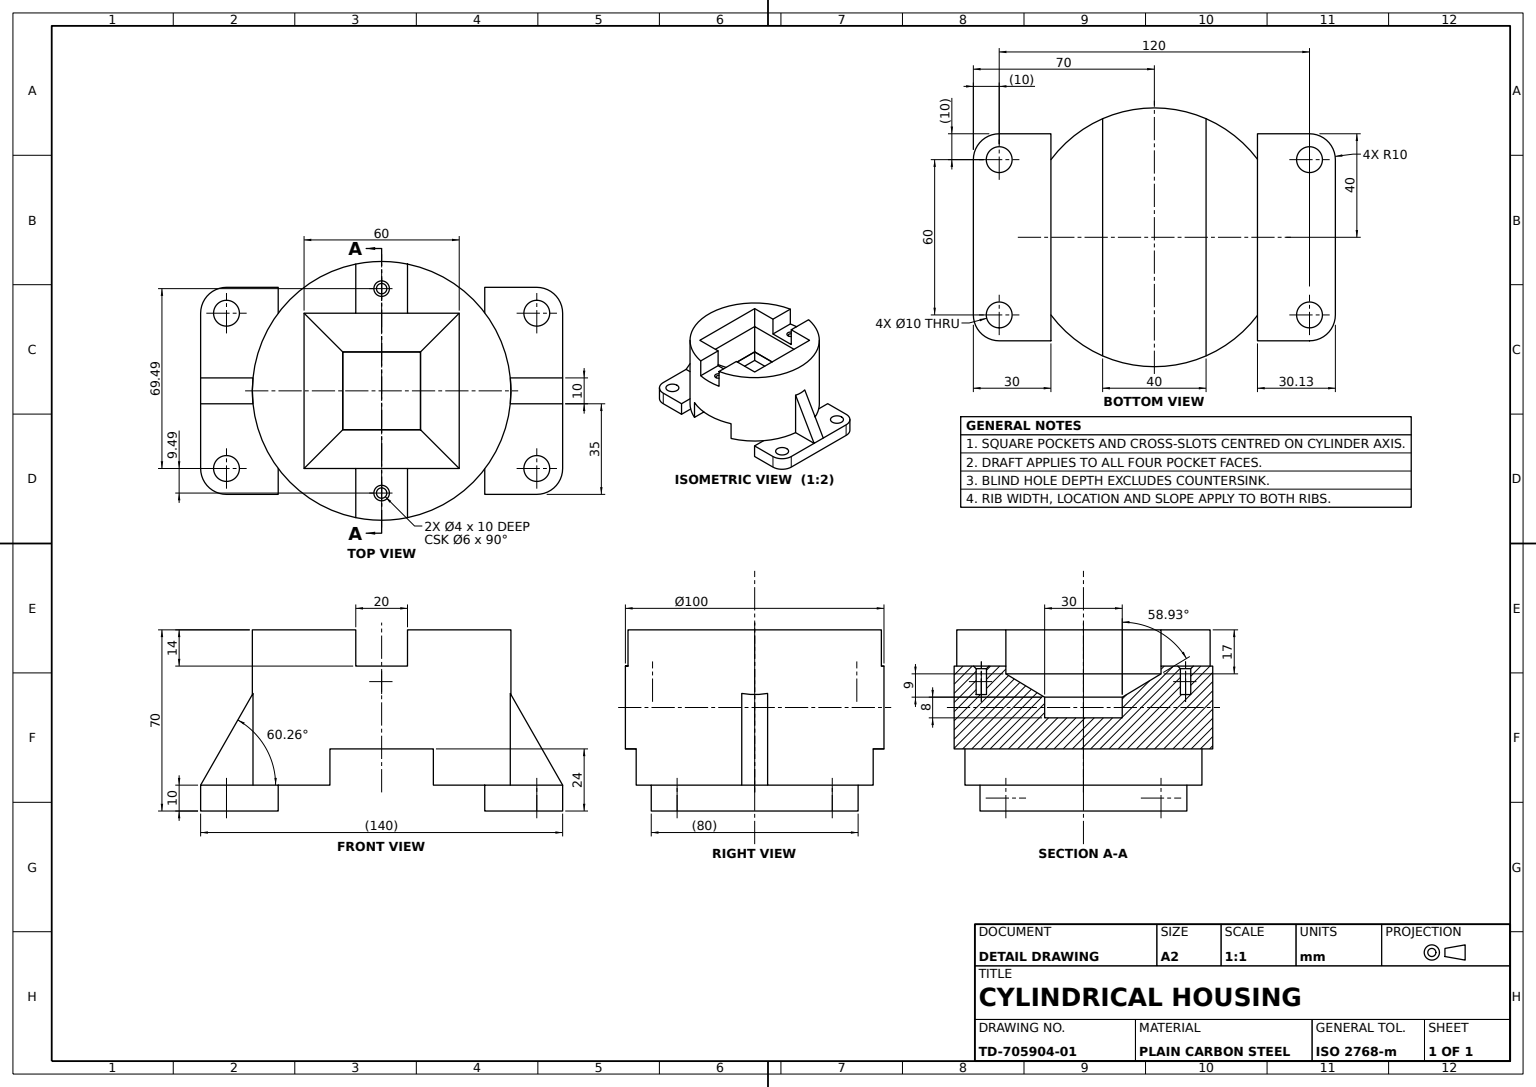
from build123d import *

# Parameters (mm, degrees)
BASE_PLATE_SKETCH_R              = 5
BASE_PLATE_DEPTH                 = 10
BODY_CYLINDER_SKETCH_R           = 50
CYLINDRICAL_BODY_100_DEPTH       = 60
SQUARE_POCKET_60X60_DEPTH        = 17
LOWER_POCKET_DEPTH               = 17
DRAFTED_BOSS_SKETCH_W            = 30
DRAFTED_BOSS_SKETCH_H            = 30
DRAFTED_BOSS_DEPTH               = 9
DRAFTED_BOSS_DRAFT               = -58.93
SLOT_A_DEPTH                     = 34
INNER_BOSS_SKETCH_W              = 60
INNER_BOSS_SKETCH_H              = 60
INNER_BOSS_DEPTH                 = 44
SLOT_B_DEPTH                     = 34
CHANNEL_CUT_DEPTH                = 17
DRAFTED_CHANNEL_SKETCH_W         = 60
DRAFTED_CHANNEL_SKETCH_H         = 60
DRAFTED_CHANNEL_CUT_DEPTH        = 9
DRAFTED_CHANNEL_CUT_DRAFT        = -58.93
STEP_POCKET_SKETCH_W             = 20
STEP_POCKET_SKETCH_H             = 20
STEP_POCKET_DEPTH                = 14
PAD_HOLE_CHAMFER_SKETCH_R        = 3
PAD_HOLE_CHAMFER_DEPTH           = 1
PAD_HOLE_CHAMFER_DRAFT           = -45
PAD_HOLE_CHAMFER_PROFILE_2_DEPTH = 1
PAD_HOLE_CHAMFER_PROFILE_2_DRAFT = -45
PAD_HOLE_SKETCH_R                = 2
PAD_HOLE_DEPTH                   = 10
LEFT_SUPPORT_RIB_REACH           = 112.905
LEFT_RIB_SKETCH_WALL_W           = 264.12201887
LEFT_RIB_SKETCH_WALL_H           = 10
RIGHT_SUPPORT_RIB_REACH          = 112.905
RIGHT_RIB_SKETCH_WALL_W          = 264.12201887
RIGHT_RIB_SKETCH_WALL_H          = 10
SIDE_CUT_A_DEPTH                 = 126
SIDE_CUT_B_DEPTH                 = 202


with BuildPart() as part:
    # Base Plate Sketch → Base Plate (new body)
    with BuildSketch(Plane(origin=(0, 0, 0), x_dir=(1, 0, 0), z_dir=(0, 1, 0))):
        with BuildLine():
            Line((-60, -40), (0, -40))
            Line((0, -40), (60, -40))
            ThreePointArc((60, -40), (67.071067812, -37.071067812), (70, -30))
            Line((70, -30), (70, 0))
            Line((70, 0), (70, 30))
            ThreePointArc((70, 30), (67.071067812, 37.071067812), (60, 40))
            Line((60, 40), (-60, 40))
            ThreePointArc((-60, 40), (-67.071067812, 37.071067812), (-70, 30))
            Line((-70, 30), (-70, -30))
            ThreePointArc((-70, -30), (-67.071067812, -37.071067812), (-60, -40))
        make_face()
        with Locations(Location((-60, -30, 0), (0, 0, 270))):
            Circle(BASE_PLATE_SKETCH_R, mode=Mode.SUBTRACT)
        with Locations(Location((60, -30, 0), (0, 0, 270))):
            Circle(BASE_PLATE_SKETCH_R, mode=Mode.SUBTRACT)
        with Locations(Location((-60, 30, 0), (0, 0, 270))):
            Circle(BASE_PLATE_SKETCH_R, mode=Mode.SUBTRACT)
        with Locations(Location((60, 30, 0), (0, 0, 270))):
            Circle(BASE_PLATE_SKETCH_R, mode=Mode.SUBTRACT)
    extrude(amount=BASE_PLATE_DEPTH)

    # Body Cylinder Sketch → Cylindrical Body Ø100 (add)
    with BuildSketch(Plane(origin=(0, 10, 0), x_dir=(1, 0, 0), z_dir=(0, 1, 0))):
        with Locations(Location((0, 0, 0), (0, 0, 53.130102354))):
            Circle(BODY_CYLINDER_SKETCH_R)
    extrude(amount=CYLINDRICAL_BODY_100_DEPTH)

    # Square Pocket Sketch → Square Pocket 60x60 (cut)
    with BuildSketch(Plane(origin=(0, 70, 0), x_dir=(1, 0, 0), z_dir=(0, 1, 0))):
        Polygon((30, 0), (30, 30), (-30, 30), (-30, -30), (30, -30), align=None)
    extrude(amount=-SQUARE_POCKET_60X60_DEPTH, mode=Mode.SUBTRACT)

    # Lower Pocket Sketch → Lower Pocket (cut)
    with BuildSketch(Plane(origin=(0, 53, 0), x_dir=(1, 0, 0), z_dir=(0, 1, 0))):
        Polygon((15, 0), (15, 15), (-15, 15), (-15, -15), (15, -15), align=None)
    extrude(amount=-LOWER_POCKET_DEPTH, mode=Mode.SUBTRACT)


with BuildPart() as body_2:
    # Drafted Boss Sketch → Drafted Boss (with draft: the straight prism first)
    with BuildSketch(Plane(origin=(0, 53, 0), x_dir=(1, 0, 0), z_dir=(0, 1, 0))):
        Rectangle(DRAFTED_BOSS_SKETCH_W, DRAFTED_BOSS_SKETCH_H)
    extrude(amount=DRAFTED_BOSS_DEPTH)
    # Drafted Boss: the draft: its side faces are tilted about the plane it starts from
    drafted_boss_sides = [body_2.faces().sort_by_distance(p)[0] for p in [
        (-15, 57.5, 0),
        (0, 57.5, 15),
        (15, 57.5, 0),
        (0, 57.5, -15),
    ]]
    draft(drafted_boss_sides, Plane(origin=(0, 53, 0), x_dir=(1, 0, 0), z_dir=(0, 1, 0)), DRAFTED_BOSS_DRAFT)


with BuildPart() as slot_a_tool:
    # Slot A Sketch → Slot A (new body)
    with BuildSketch(Plane(origin=(0, 62, 0), x_dir=(1, 0, 0), z_dir=(0, 1, 0))):
        Polygon((15, 0), (15, 15), (-15, 15), (-15, -15), (15, -15), align=None)
    extrude(amount=-SLOT_A_DEPTH)


with BuildPart() as part_1:
    add(part.part)

    # Slot A: cut by slot_a_tool
    add(slot_a_tool.part, mode=Mode.SUBTRACT)



with BuildPart() as body_2_1:
    add(body_2.part)

    # Slot A: cut by slot_a_tool
    add(slot_a_tool.part, mode=Mode.SUBTRACT)


with BuildPart() as part_2:
    add(part_1.part)

    add(body_2_1.part)  # Inner Boss merges body 2
    # Inner Boss Sketch → Inner Boss (add)
    with BuildSketch(Plane(origin=(0, 70, 0), x_dir=(1, 0, 0), z_dir=(0, 1, 0))):
        Rectangle(INNER_BOSS_SKETCH_W, INNER_BOSS_SKETCH_H)
    extrude(amount=-INNER_BOSS_DEPTH)

    # Slot B Sketch → Slot B (cut)
    with BuildSketch(Plane(origin=(0, 70, 0), x_dir=(1, 0, 0), z_dir=(0, 1, 0))):
        Polygon((15, 0), (15, 15), (-15, 15), (-15, -15), (15, -15), align=None)
    extrude(amount=-SLOT_B_DEPTH, mode=Mode.SUBTRACT)

    # Channel Sketch → Channel Cut (cut)
    with BuildSketch(Plane(origin=(0, 70, 0), x_dir=(1, 0, 0), z_dir=(0, 1, 0))):
        Polygon((30, 0), (30, 30), (-30, 30), (-30, -30), (30, -30), align=None)
    extrude(amount=-CHANNEL_CUT_DEPTH, mode=Mode.SUBTRACT)


with BuildPart() as drafted_channel_cut_tool:
    # Drafted Channel Sketch → Drafted Channel Cut (with draft: the straight prism first)
    with BuildSketch(Plane(origin=(0, 53, 0), x_dir=(1, 0, 0), z_dir=(0, 1, 0))):
        Rectangle(DRAFTED_CHANNEL_SKETCH_W, DRAFTED_CHANNEL_SKETCH_H)
    extrude(amount=-DRAFTED_CHANNEL_CUT_DEPTH)
    # Drafted Channel Cut: the draft: its side faces are tilted about the plane it starts from
    drafted_channel_cut_sides = [drafted_channel_cut_tool.faces().sort_by_distance(p)[0] for p in [
        (-30, 48.5, 0),
        (0, 48.5, 30),
        (30, 48.5, 0),
        (0, 48.5, -30),
    ]]
    draft(drafted_channel_cut_sides, Plane(origin=(0, 53, 0), x_dir=(1, 0, 0), z_dir=(0, 1, 0)), DRAFTED_CHANNEL_CUT_DRAFT)


with BuildPart() as part_3:
    add(part_2.part)

    # Drafted Channel Cut: cut by drafted_channel_cut_tool
    add(drafted_channel_cut_tool.part, mode=Mode.SUBTRACT)

    # Step Pocket Sketch → Step Pocket (cut)
    with BuildSketch(Plane(origin=(0, 70, 0), x_dir=(1, 0, 0), z_dir=(0, 1, 0))):
        with Locations((0, -40)):
            Rectangle(STEP_POCKET_SKETCH_W, STEP_POCKET_SKETCH_H)
        Polygon((0, 30), (10, 30), (10, 50), (-10, 50), (-10, 30), align=None)
    extrude(amount=-STEP_POCKET_DEPTH, mode=Mode.SUBTRACT)


with BuildPart() as pad_hole_chamfer_tool:
    # Pad Hole Chamfer Sketch → Pad Hole Chamfer (with draft: the straight prism first)
    with BuildSketch(Plane(origin=(0, 56, 0), x_dir=(1, 0, 0), z_dir=(0, 1, 0))):
        with Locations((0, -39.494897428)):
            Circle(PAD_HOLE_CHAMFER_SKETCH_R)
    extrude(amount=-PAD_HOLE_CHAMFER_DEPTH)
    # Pad Hole Chamfer: the draft: its side faces are tilted about the plane it starts from
    pad_hole_chamfer_sides = [pad_hole_chamfer_tool.faces().sort_by_distance(p)[0] for p in [
        (-3, 55.5, 39.494897428),
    ]]
    draft(pad_hole_chamfer_sides, Plane(origin=(0, 56, 0), x_dir=(1, 0, 0), z_dir=(0, 1, 0)), PAD_HOLE_CHAMFER_DRAFT)


with BuildPart() as part_4:
    add(part_3.part)

    # Pad Hole Chamfer: cut by pad_hole_chamfer_tool
    add(pad_hole_chamfer_tool.part, mode=Mode.SUBTRACT)


with BuildPart() as pad_hole_chamfer_profile_2_tool:
    # Pad Hole Chamfer Sketch → Pad Hole Chamfer profile 2 (with draft: the straight prism first)
    with BuildSketch(Plane(origin=(0, 56, 0), x_dir=(1, 0, 0), z_dir=(0, 1, 0))):
        with Locations((0, 39.494897428)):
            Circle(PAD_HOLE_CHAMFER_SKETCH_R)
    extrude(amount=-PAD_HOLE_CHAMFER_PROFILE_2_DEPTH)
    # Pad Hole Chamfer profile 2: the draft: its side faces are tilted about the plane it starts from
    pad_hole_chamfer_profile_2_sides = [pad_hole_chamfer_profile_2_tool.faces().sort_by_distance(p)[0] for p in [
        (-3, 55.5, -39.494897428),
    ]]
    draft(pad_hole_chamfer_profile_2_sides, Plane(origin=(0, 56, 0), x_dir=(1, 0, 0), z_dir=(0, 1, 0)), PAD_HOLE_CHAMFER_PROFILE_2_DRAFT)


with BuildPart() as part_5:
    add(part_4.part)

    # Pad Hole Chamfer profile 2: cut by pad_hole_chamfer_profile_2_tool
    add(pad_hole_chamfer_profile_2_tool.part, mode=Mode.SUBTRACT)

    # Pad Hole Sketch → Pad Hole (cut)
    with BuildSketch(Plane(origin=(0, 55, 0), x_dir=(1, 0, 0), z_dir=(0, 1, 0))):
        with Locations(Location((0, 39.494897428, 0), (0, 0, 270))):
            Circle(PAD_HOLE_SKETCH_R)
        with Locations(Location((0, -39.494897428, 0), (0, 0, 270))):
            Circle(PAD_HOLE_SKETCH_R)
    extrude(amount=-PAD_HOLE_DEPTH, mode=Mode.SUBTRACT)

    # Left Rib Sketch wall → Left Support Rib (add, up to next)
    with BuildSketch(Plane(origin=(-60, 27.5, 0), x_dir=(-0.496138938357, -0.868243142124, 0), z_dir=(0.868243142124, -0.496138938357, 0)), mode=Mode.PRIVATE) as left_support_rib_sk1:
        Rectangle(LEFT_RIB_SKETCH_WALL_W, LEFT_RIB_SKETCH_WALL_H)
    left_support_rib_tool1 = extrude(left_support_rib_sk1.sketch, amount=LEFT_SUPPORT_RIB_REACH, mode=Mode.PRIVATE) - part_5.part
    add(left_support_rib_tool1.solids().sort_by_distance((-60, 27.5, 0))[0])

    # Right Rib Sketch wall → Right Support Rib (add, up to next)
    with BuildSketch(Plane(origin=(60, 27.5, 0), x_dir=(0.496138938357, -0.868243142124, 0), z_dir=(0.868243142124, 0.496138938357, 0)), mode=Mode.PRIVATE) as right_support_rib_sk1:
        Rectangle(RIGHT_RIB_SKETCH_WALL_W, RIGHT_RIB_SKETCH_WALL_H)
    right_support_rib_tool1 = extrude(right_support_rib_sk1.sketch, amount=-RIGHT_SUPPORT_RIB_REACH, mode=Mode.PRIVATE) - part_5.part
    add(right_support_rib_tool1.solids().sort_by_distance((60, 27.5, 0))[0])

    # Side Cut A Sketch → Side Cut A (cut)
    with BuildSketch(Plane.XY.offset(50)):
        Polygon((0, 10), (-40, 10), (-40, 0), (39.874685928, 0), (39.874685928, 10), align=None)
    extrude(amount=-SIDE_CUT_A_DEPTH, mode=Mode.SUBTRACT)

    # Side Cut B Sketch → Side Cut B (cut)
    with BuildSketch(Plane.XY.offset(50)):
        Polygon((0, 0), (20, 0), (20, 24), (-20, 24), (-20, 0), align=None)
    extrude(amount=-SIDE_CUT_B_DEPTH, mode=Mode.SUBTRACT)


solid = part_5.part
